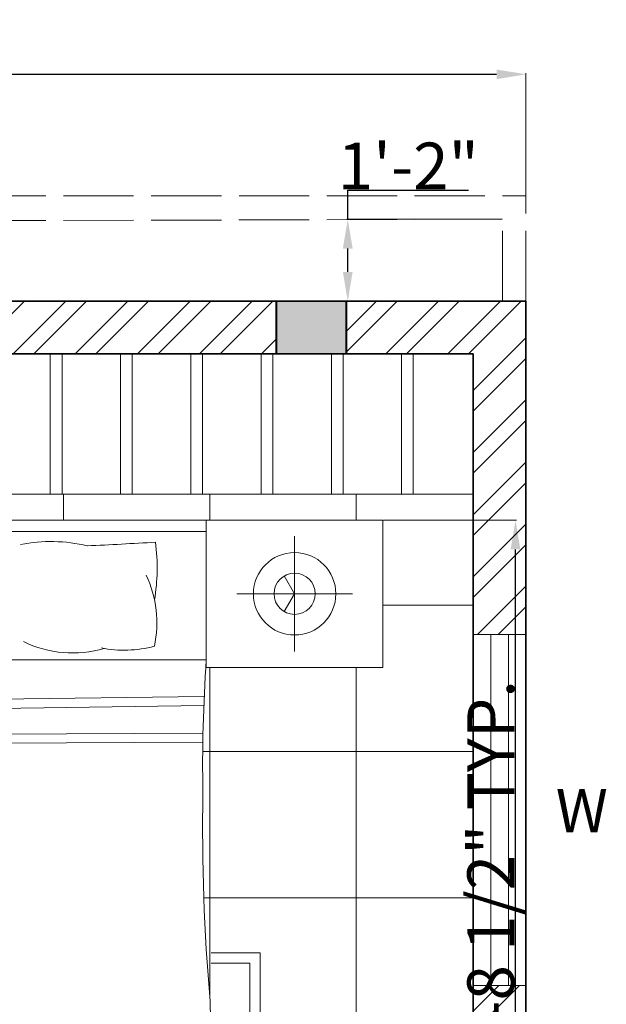
# Model space of a CAD drawing. Units: inches. Extents: x 351 to 1738, y -265 to 286.
# Tile 37 of 38: x 1480 to 1580, y 118 to 286. Entities that reach past the tile are written whole.
import ezdxf

# ---------------------------------------------------------------- set-up
doc = ezdxf.new("R2010")
doc.units = ezdxf.units.IN
doc.header["$MEASUREMENT"] = 0
doc.linetypes.add('ACAD_ISO02W100', pattern=[15, 12, -3])
for name, color, linetype, lineweight in [('A-ANNO-DIMS', 2, 'Continuous', 18), ('A-ANNO-SYMB', 7, 'Continuous', 18), ('A-COLS', 7, 'Continuous', 40), ('A-COLS-PATT', 6, 'Continuous', 13), ('A-FLOR-CASE', 9, 'Continuous', 18), ('A-FLOR-OVHD', 1, 'ACAD_ISO02W100', 18), ('A-FLOR-PATT', 9, 'Continuous', 9), ('A-FURN', 18, 'Continuous', 13), ('A-GLAZ', 4, 'Continuous', 18), ('A-WALL', 7, 'Continuous', 35), ('A-WALL-PATT', 152, 'Continuous', 13)]:
    doc.layers.add(name, color=color, linetype=linetype, lineweight=lineweight)
doc.styles.add('Annotative', font='arial.ttf')
doc.styles.get("Standard").update_dxf_attribs({"font": 'arial.ttf'})
doc.dimstyles.get("Standard").update_dxf_attribs({"dimtxt": 8, "dimasz": 5, "dimexe": 0.18, "dimexo": 0.0625, "dimgap": 0.09, "dimtad": 1, "dimtoh": 1, "dimzin": 0, "dimdsep": 46, "dimlunit": 4, "dimtxsty": 'Standard', "dimcen": 0, "dimclre": 256, "dimadec": 0, "dimazin": 0, "dimtfac": 1, "dimtofl": 0, "dimtmove": 0, "dimatfit": 3, "dimfxl": 1, "dimtolj": 1, "dimtzin": 0, "dimlwe": -1, "dimarcsym": 0})

# ---------------------------------------------------------------- blocks, each defined once
blk = doc.blocks.new('*D7')
at = {"layer": 'A-ANNO-DIMS', "color": 0, "transparency": 16777216}
for p, q in [((1034.7, 256.03), (1034.7, 276.92)), ((1566.7, 256.03), (1566.7, 276.92))]:
    blk.add_line(p, q, dxfattribs=at)
at = {"layer": 'A-ANNO-DIMS', "color": 0, "lineweight": -2, "transparency": 16777216}
blk.add_line((1039.7, 276.74), (1561.7, 276.74), dxfattribs=at)
at = {"layer": 'A-ANNO-DIMS', "color": 0, "transparency": 16777216}
for points in [[(1039.7, 277.57), (1039.7, 275.91), (1034.7, 276.74)], [(1561.7, 277.57), (1561.7, 275.91), (1566.7, 276.74)]]:
    blk.add_solid(points, dxfattribs=at)
at = {"layer": 'Defpoints', "color": 0, "transparency": 16777216}
for p in [(1566.7, 276.74), (1034.7, 255.96), (1566.7, 255.96)]:
    blk.add_point(p, dxfattribs=at)
at = {"layer": 'A-ANNO-DIMS', "color": 0, "transparency": 16777216, "insert": (1300.7, 280.83), "char_height": 8, "attachment_point": 5}
blk.add_mtext('\\A1;44\'-4"', dxfattribs=at)
blk = doc.blocks.new('*D9')
at = {"layer": 'A-ANNO-DIMS', "color": 0, "lineweight": -2, "transparency": 16777216}
for p, q in [((1536.28, 251.96), (1536.28, 256.96)), ((1536.28, 256.96), (1556.88, 256.96)), ((1536.28, 242.96), (1536.28, 246.96))]:
    blk.add_line(p, q, dxfattribs=at)
at = {"layer": 'A-ANNO-DIMS', "color": 0, "transparency": 16777216}
for p, q in [((1562.64, 251.96), (1536.1, 251.96)), ((1562.64, 237.96), (1536.1, 237.96))]:
    blk.add_line(p, q, dxfattribs=at)
for points in [[(1535.44, 246.96), (1537.11, 246.96), (1536.28, 251.96)], [(1535.44, 242.96), (1537.11, 242.96), (1536.28, 237.96)]]:
    blk.add_solid(points, dxfattribs=at)
at = {"layer": 'Defpoints', "color": 0, "transparency": 16777216}
for p in [(1536.28, 251.96), (1562.7, 251.96), (1562.7, 237.96)]:
    blk.add_point(p, dxfattribs=at)
at = {"layer": 'A-ANNO-DIMS', "color": 0, "transparency": 16777216, "insert": (1546.62, 261.07), "char_height": 8, "attachment_point": 5}
blk.add_mtext('\\A1;1\'-2"', dxfattribs=at)
blk = doc.blocks.new('BED-DOUBLE-W-NIGHTSTANDS')
for p, q in [((120.72, 126.39), (30.18, 126.39)), ((135.81, 105.9), (135.81, 125.61)), ((125.95, 115.76), (145.67, 115.76)), ((30.18, 104.48), (120.72, 104.48)), ((120.32, 98.22), (66.59, 97.46)), ((120.26, 96.67), (65.46, 95.89)), ((120.18, 91.92), (62.88, 91.69)), ((120.19, 90.37), (62.29, 90.13))]:
    blk.add_line(p, q)
for points in [[(30.18, 103.18), (0, 103.18), (0, 128.33), (150.9, 128.33), (150.9, 103.18), (120.72, 103.18), (120.72, 128.33)], [(134.05, 118.81), (135.81, 115.76), (134.05, 112.71)], [(121.56, 54.36), (129.93, 54.36), (129.93, 0), (19.92, 0), (19.92, 54.36), (28.45, 54.36)], [(28.45, 52.61), (21.67, 52.61), (21.67, 1.75), (128.18, 1.75), (128.18, 52.61), (121.53, 52.61)]]:
    blk.add_lwpolyline(points)
for points in [[(112.05, 124.57, -0.074897), (111.87, 114.71, 0.472817)], [(121.36, 46.14, 0.056112), (122.46, 37.83, 0.095341), (124.58, 29.84)]]:
    blk.add_lwpolyline(points, format="xyb")
for radius in [7.04, 3.52]:
    blk.add_circle((135.81, 115.76), radius)
for centre, radius, start, end in [((94.14, 98.17), 26.53, 76.3427, 101.1841), ((28.88, 1560.65), 1438.48, 272.85022, 273.31479), ((92.83, 110.76), 19.45, 348.2417, 24.8684), ((97.94, 124.85), 19.21, 243.8761, 286.1746), ((106.67, 126.34), 20.22, 258.9631, 284.8961), ((391.24, 86.04), 271.14, 176.1, 180.9282), ((473.78, 76.18), 353.69, 179.1145, 184.8735)]:
    blk.add_arc(centre, radius, start, end)
blk = doc.blocks.new('WARDROBE-PANELLED')
for p, q in [((101.27, 24), (101.27, 0)), ((103.27, 24), (103.27, 0)), ((113.27, 24), (113.27, 0)), ((115.27, 24), (115.27, 0)), ((125.27, 24), (125.27, 0)), ((127.27, 24), (127.27, 0)), ((137.27, 24), (137.27, 0)), ((139.27, 24), (139.27, 0)), ((149.27, 24), (149.27, 0)), ((151.27, 24), (151.27, 0)), ((161.27, 24), (161.27, 0)), ((163.27, 24), (163.27, 0)), ((0, 0), (173.5, 0))]:
    blk.add_line(p, q)
blk = doc.blocks.new('WIN-60')
for p, q in [((0, 6), (60, 6)), ((0, 3), (60, 3))]:
    blk.add_line(p, q)
blk.add_lwpolyline([(60, 0), (60, 9), (0, 9), (0, 0)], close=True)
blk = doc.blocks.new('*D47')
at = {"layer": 'A-ANNO-DIMS', "transparency": 16777216}
for p, q in [((1542.36, 200.52), (1565.11, 200.52)), ((1542.36, 72.19), (1565.11, 72.19))]:
    blk.add_line(p, q, dxfattribs=at)
at = {"layer": 'A-ANNO-DIMS', "color": 0, "lineweight": -2, "transparency": 16777216}
blk.add_line((1564.93, 77.19), (1564.93, 195.52), dxfattribs=at)
at = {"layer": 'A-ANNO-DIMS', "color": 0, "transparency": 16777216}
for points in [[(1564.1, 195.52), (1565.76, 195.52), (1564.93, 200.52)], [(1564.1, 77.19), (1565.76, 77.19), (1564.93, 72.19)]]:
    blk.add_solid(points, dxfattribs=at)
at = {"layer": 'Defpoints', "color": 0, "transparency": 16777216}
for p in [(1542.29, 200.52), (1564.93, 200.52), (1542.29, 72.19)]:
    blk.add_point(p, dxfattribs=at)
at = {"layer": 'A-ANNO-DIMS', "color": 0, "transparency": 16777216, "insert": (1560.7, 136.35), "char_height": 8, "attachment_point": 5, "rotation": 90}
blk.add_mtext('\\A1;10\'-8 1/2" TYP.', dxfattribs=at)

msp = doc.modelspace()

# ---------------------------------------------------------------- hatches: boundary and pattern name
at = {"layer": 'A-COLS-PATT'}
h = msp.add_hatch(color=256, dxfattribs=at)
h.dxf.hatch_style = 1
h.paths.add_polyline_path([(1112.704, 237.963), (1103.704, 237.963), (1103.704, 228.963), (1112.704, 228.963)])
h.paths.add_polyline_path([(1115.704, 237.963), (1112.704, 237.963), (1112.704, 228.963), (1115.704, 228.963)])
h.paths.add_polyline_path([(1043.704, 255.963), (1034.704, 255.963), (1034.704, 243.963), (1043.704, 243.963)])
h.paths.add_polyline_path([(1043.704, 210.963), (1034.704, 210.963), (1034.704, 198.963), (1043.704, 198.963)])
h.paths.add_polyline_path([(1043.704, -45.037), (1034.704, -45.037), (1034.704, -57.037), (1043.704, -57.037)])
h.paths.add_polyline_path([(1112.704, -45.037), (1103.704, -45.037), (1103.704, -57.037), (1112.704, -57.037)])
h.paths.add_polyline_path([(1112.704, -161.037), (1103.704, -161.037), (1103.704, -164.037), (1103.704, -173.037), (1112.704, -173.037)])
h.paths.add_polyline_path([(1043.704, -161.037), (1034.704, -161.037), (1034.704, -173.037), (1043.704, -173.037)])
h.paths.add_polyline_path([(1248.549, -164.037), (1236.549, -164.037), (1236.549, -173.037), (1248.549, -173.037)])
h.paths.add_polyline_path([(1248.549, -50), (1236.549, -50), (1236.549, -59), (1248.549, -59)])
h.paths.add_polyline_path([(1248.704, 73.463), (1244.704, 73.463), (1244.704, 64.463), (1248.704, 64.463)])
h.paths.add_polyline_path([(1244.704, 73.463), (1236.704, 73.463), (1236.704, 64.463), (1244.704, 64.463)])
h.paths.add_polyline_path([(1248.704, 237.963), (1236.704, 237.963), (1236.704, 228.963), (1248.704, 228.963)])
h.paths.add_polyline_path([(1392.204, 237.963), (1380.204, 237.963), (1380.204, 228.963), (1392.204, 228.963)])
h.paths.add_polyline_path([(1536.064, 237.963), (1524.064, 237.963), (1524.064, 228.963), (1536.064, 228.963)])
h.paths.add_polyline_path([(1536.064, 73.463), (1524.064, 73.463), (1524.064, 64.463), (1536.064, 64.463)])
h.paths.add_polyline_path([(1384.204, 73.463), (1380.204, 73.463), (1380.204, 64.463), (1384.204, 64.463)])
h.paths.add_polyline_path([(1392.064, 73.463), (1384.204, 73.463), (1384.204, 64.463), (1392.064, 64.463)])
h.paths.add_polyline_path([(1536.064, -53.037), (1524.064, -53.037), (1524.064, -57.037), (1536.064, -57.037)])
h.paths.add_polyline_path([(1536.064, -48.037), (1524.064, -48.037), (1524.064, -53.037), (1536.064, -53.037)])
h.paths.add_polyline_path([(1392.064, -48.037), (1380.064, -48.037), (1380.064, -56.5), (1380.065, -57.037), (1392.064, -57.037)])
h.paths.add_polyline_path([(1536.064, -164.037), (1524.064, -164.037), (1524.064, -173.037), (1536.064, -173.037)])
at = {"layer": 'A-FLOR-PATT', "transparency": 33554559}
h = msp.add_hatch(dxfattribs=at)
h.set_pattern_fill('ANSI37', color=256, scale=200, angle=135)
h.set_pattern_definition([(180, (1112.704, -164.037), (-2e-15, -25), []), (270, (1112.704, -164.037), (25, -5e-15), [])])
h.paths.add_polyline_path([(1380.064, 73.463), (1380.132, 148.463), (1338.064, 148.463), (1290.704, 148.463), (1290.704, 88.463), (1248.704, 88.463), (1248.704, -2.009), (1244.704, -2.009), (1244.704, 142.457), (1160.704, 142.457), (1160.704, 158.963), (1160.704, 170.137), (1160.704, 206.137), (1160.704, 228.963), (1112.704, 228.963), (1112.704, 209.963), (1112.704, 168.963), (1124.704, 168.963), (1124.704, 162.963), (1112.704, 162.963), (1112.704, 64.463), (1112.704, 60.463), (1112.704, 0.463), (1112.704, -48.026), (1146.804, -47.981), (1146.804, -35.691), (1207.804, -35.691), (1207.804, -47.902), (1236.542, -47.864), (1236.544, -50.009), (1248.5, -50.009), (1248.506, -102.915), (1248.512, -150.915), (1248.514, -164.037), (1248.549, -164.037), (1273.017, -164.037), (1273.017, -128.799), (1355.24, -128.799), (1355.24, -164.037), (1384.204, -164.037), (1384.204, -57.037), (1380.064, -57.037), (1380.064, -48.037), (1392.064, -48.037), (1392.064, -53.037), (1406.549, -53.037), (1406.549, -57.037), (1401.204, -57.037), (1401.204, -147.037), (1468.204, -147.037), (1468.204, -138.5), (1472.204, -138.5), (1472.204, -102.5), (1468.204, -102.5), (1468.204, -57.037), (1442.549, -57.037), (1442.549, -53.037), (1463.049, -53.037), (1463.049, -40.747), (1524.049, -40.747), (1524.049, -48.037), (1536.064, -48.037), (1536.064, -53.037), (1557.704, -53.037), (1557.704, 204.963), (1384.204, 204.963), (1384.204, 73.463), (1392.064, 73.463), (1392.064, 64.463), (1384.204, 64.463), (1384.204, -3.5), (1380.204, -3.537), (1380.204, 64.463), (1380.064, 64.463)])
h.paths.add_polyline_path([(1510.714, 86.458, -0.1039845), (1511.661, 85.595, 0.4704384), (1510.158, 87.614, 0.0961001)], flags=16)
h.paths.add_polyline_path([(1510.443, 100.266, 0.009798), (1504.693, 100.48, 0.0287898), (1504.6, 99.767, -0.1653311), (1505.519, 96.135, -0.1436014)], flags=16)
h.paths.add_polyline_path([(1487.201, 85.595, -0.1039845), (1488.148, 86.458, 0.0961001), (1488.704, 87.614, 0.4704384)], flags=0)
h.paths.add_polyline_path([(1495.052, 100.43), (1494.178, 100.43, -0.0264629), (1494.262, 99.774, -0.1442193)], flags=16)
h.paths.add_polyline_path([(1444.485, 86.458, -0.1039845), (1445.433, 85.595, 0.4704384), (1443.93, 87.614, 0.0961001)], flags=16)
h.paths.add_polyline_path([(1420.972, 85.595, -0.1039845), (1421.92, 86.458, 0.0961001), (1422.475, 87.614, 0.4704384)], flags=16)
h.paths.add_polyline_path([(1428.632, 100.335, 0.0010541), (1427.971, 100.309, -0.0215241), (1428.033, 99.774, -0.1143008)], flags=16)
h.paths.add_polyline_path([(1419.906, 143.708, 0.0249793), (1420.222, 157.526), (1421.573, 159.101), (1421.573, 175.369), (1391.393, 175.369), (1391.393, 200.519), (1542.294, 200.519), (1542.294, 175.369), (1512.028, 175.369, 0.0198653), (1511.521, 153.838, 0.0251335), (1512.758, 118.323, 0.0205529), (1512.942, 115.253), (1419.834, 115.253, -0.0004142), (1419.843, 124.798), (1413.059, 124.798), (1413.059, 84.437, -0.0618528), (1415.831, 80.45, -0.0930773), (1420.972, 85.595, -0.2675367), (1422.371, 84.732, 0.0851103), (1424.052, 84.616, -0.8853927), (1424.033, 84.851, -1.1258145), (1424.073, 84.366, -0.0879871), (1422.371, 84.732, -0.2675367), (1422.326, 83.089, -0.3705421), (1420.972, 85.595, 0.0930773), (1415.831, 80.45, -0.0874142), (1417.914, 73.937), (1418.941, 73.937, 0.0272504), (1418.913, 76.906, -0.1157032), (1421.051, 73.937), (1445.354, 73.937, -0.1157032), (1447.492, 76.906, 0.0272504), (1447.464, 73.937), (1448.491, 73.937, -0.0874142), (1450.574, 80.45, 0.0930773), (1445.433, 85.595, -0.3705421), (1444.079, 83.089, -0.2675367), (1444.034, 84.732, -0.0879871), (1442.332, 84.366, -1.1258145), (1442.372, 84.851, -2.0327363), (1442.364, 84.368, 0.0863779), (1444.034, 84.732, -0.2675367), (1445.433, 85.595, -0.0930773), (1450.574, 80.45, -0.2577317), (1466.483, 90.927, -0.4786702), (1468.832, 91.907, -0.4786702), (1471.18, 90.927, -0.26264), (1483.053, 81.78, -0.0718662), (1487.201, 85.595, -0.2675367), (1488.6, 84.732, 0.0851103), (1490.28, 84.616, -0.8853927), (1490.262, 84.851, -1.1258145), (1490.301, 84.366, -0.0879871), (1488.6, 84.732, -0.2675367), (1488.554, 83.089, -0.3705421), (1487.201, 85.595, 0.0718662), (1483.053, 81.78, -0.1320648), (1484.143, 73.937), (1485.169, 73.937, 0.0272504), (1485.142, 76.906, -0.1157032), (1487.28, 73.937), (1511.582, 73.937, -0.1157032), (1513.72, 76.906, 0.0272504), (1513.693, 73.937), (1514.719, 73.937, -0.0874142), (1516.802, 80.45, 0.0930773), (1511.661, 85.595, -0.3705421), (1510.308, 83.089, -0.2675367), (1510.262, 84.732, -0.0879871), (1508.561, 84.366, -1.1258145), (1508.601, 84.851, -2.0327363), (1508.592, 84.368, 0.0863779), (1510.262, 84.732, -0.2675367), (1511.661, 85.595, -0.0930773), (1516.802, 80.45, -0.0618528), (1519.575, 84.437), (1519.575, 73.937), (1413.059, 73.937), (1413.059, 124.798), (1419.843, 124.798, -0.0008205)], flags=16)
h.paths.add_polyline_path([(1220.149, 54.133, -0.1039845), (1220.869, 53.476, 0.4704384), (1219.727, 55.011, 0.0961001)], flags=16)
h.paths.add_polyline_path([(1219.944, 64.626, 0.009798), (1215.574, 64.789, 0.0287898), (1215.503, 64.247, -0.1653311), (1216.201, 61.487, -0.1436014)], flags=16)
h.paths.add_polyline_path([(1209.779, 64.449, 0.0974459), (1209.339, 64.751), (1208.247, 64.751, 0.1273905), (1207.7, 64.326, 0.1715858), (1206.95, 61.475, -0.1588542), (1207.636, 59.45, 0.0158984), (1207.795, 59.218, 0.0615457), (1208.598, 59.616, 0.1754158), (1208.638, 60.099, -0.2847793), (1209.348, 62.472, 0.3262165)], flags=16)
h.paths.add_polyline_path([(1169.818, 54.133, -0.1039845), (1170.538, 53.476, 0.4704384), (1169.396, 55.011, 0.0961001)], flags=16)
h.paths.add_polyline_path([(1159.017, 62.472, 0.2847642), (1158.307, 60.099, -0.1754332), (1158.267, 59.616, 0.3929302), (1159.448, 64.449, -0.3262298)], flags=16)
h.paths.add_polyline_path([(1156.342, 58.239, -0.1783213), (1154.011, 55.31, -0.1747359), (1154.722, 55.233, -0.2008015), (1156.27, 56.086, 0.1269899), (1157.283, 58.991, -0.0912053)], flags=16)
h.paths.add_polyline_path([(1156.624, 61.413, 0.1572752), (1157.316, 64.247, 0.1696217)], flags=16)
h.paths.add_polyline_path([(1152.67, 54.133, -0.0961001), (1151.95, 53.476, 0.0640762), (1154.465, 54.384, 0.1990158)], flags=16)
h.paths.add_polyline_path([(1202.281, 53.476, -0.1039845), (1203, 54.133, 0.0961001), (1203.423, 55.011, 0.4704384)], flags=0)
h.paths.add_polyline_path([(1151.139, 97.64, 0.0249793), (1151.379, 108.141), (1152.406, 109.338), (1152.406, 121.701), (1129.47, 121.701), (1129.47, 140.814), (1244.149, 140.814), (1244.149, 121.701), (1221.148, 121.701, 0.0198653), (1220.763, 105.338, 0.0251335), (1221.703, 78.349, 0.0205529), (1221.843, 76.016), (1151.078, 76.016, -0.1287433), (1148.786, 65.037, 0.5393525), (1150.327, 64.171, -0.027594), (1163.481, 64.751, 0.0976954), (1163.04, 64.449, 0.3262165), (1163.471, 62.472, -0.2847765), (1164.181, 60.099, -0.1947567), (1165.846, 61.443, -0.1554021), (1165.172, 64.247, -0.1660224), (1165.869, 61.475, -0.1770142), (1167.852, 62.77, -0.4482027), (1169.974, 60.807, -0.3934987), (1167.679, 57.86, -0.8955483), (1168.438, 54.524, -0.3557668), (1166.218, 56.086, -0.066024), (1165.505, 57.539), (1165.251, 56.243, -0.3717324), (1164.02, 59.758, -0.3736141), (1163.04, 64.449, -0.0976954), (1163.481, 64.751, 0.0213538), (1153.294, 64.429, -0.1341826), (1156.695, 61.368, 0.1868727), (1154.636, 62.77, 0.4482027), (1152.514, 60.807, 0.4037263), (1154.905, 57.846, 0.7112192), (1153.334, 55, 0.5315397), (1151.95, 53.476, -0.2675367), (1153.013, 52.821, 0.0851103), (1154.29, 52.732, -0.8853927), (1154.276, 52.911, -1.1258145), (1154.306, 52.543, -0.0879871), (1153.013, 52.821, -0.2675367), (1152.978, 51.572, -0.3705421), (1151.95, 53.476, 0.0930773), (1148.043, 49.566, -0.0874142), (1149.626, 44.617), (1150.406, 44.617, 0.0272504), (1150.385, 46.873, -0.1157032), (1152.01, 44.617), (1170.478, 44.617, -0.1157032), (1172.103, 46.873, 0.0272504), (1172.082, 44.617), (1172.862, 44.617, -0.0874142), (1174.445, 49.566, 0.0930773), (1170.538, 53.476, -0.3705421), (1169.51, 51.572, -0.2675367), (1169.475, 52.821, -0.0879871), (1168.182, 52.543, -1.1258145), (1168.212, 52.911, -2.0327363), (1168.206, 52.544, 0.0863779), (1169.475, 52.821, -0.2675367), (1170.538, 53.476, -0.0930773), (1174.445, 49.566, -0.2577317), (1186.536, 57.528, -0.4786702), (1188.321, 58.273, -0.4786702), (1190.106, 57.528, -0.26264), (1199.128, 50.577, -0.0718662), (1202.281, 53.476, -0.2675367), (1203.344, 52.821, 0.0851103), (1204.621, 52.732, -0.8853927), (1204.607, 52.911, -1.1258145), (1204.637, 52.543, -0.0879871), (1203.344, 52.821, -0.2675367), (1203.309, 51.572, -0.3705421), (1202.281, 53.476, 0.0718662), (1199.128, 50.577, -0.1320648), (1199.957, 44.617), (1200.737, 44.617, 0.0272504), (1200.716, 46.873, -0.1157032), (1202.341, 44.617), (1220.809, 44.617, -0.1157032), (1222.434, 46.873, 0.0272504), (1222.413, 44.617), (1223.193, 44.617, -0.0874142), (1224.776, 49.566, 0.0930773), (1220.869, 53.476, -0.3705421), (1219.841, 51.572, -0.2675367), (1219.806, 52.821, -0.0879871), (1218.513, 52.543, -1.1258145), (1218.543, 52.911, -2.0327363), (1218.537, 52.544, 0.0863779), (1219.806, 52.821, -0.2675367), (1220.869, 53.476, -0.0930773), (1224.776, 49.566, -0.0618528), (1226.883, 52.597), (1226.883, 44.617), (1145.936, 44.617), (1145.936, 83.269), (1151.091, 83.269, -0.0008205)], flags=16)
h.paths.add_polyline_path([(1218.01, 57.86, -0.8955483), (1218.769, 54.524, -0.3557668), (1216.549, 56.086, -0.066024), (1215.836, 57.539), (1215.582, 56.243, -0.3717324), (1214.351, 59.758, -0.3736141), (1213.371, 64.449, 0.3262165), (1213.802, 62.472, -0.2847765), (1214.512, 60.099, -0.1947567), (1216.177, 61.443, -0.1799907), (1218.183, 62.77, -0.4482027), (1220.305, 60.807, -0.3934987)], flags=16)
h.paths.add_polyline_path([(1424.735, 91.363, -0.3934987), (1421.715, 95.241, -0.4482027), (1424.507, 97.824, -0.1799907), (1427.147, 96.077, -0.1947567), (1429.338, 94.309, -0.2847765), (1430.272, 97.432, 0.3262165), (1430.839, 100.034, -0.3736141), (1429.55, 93.861, -0.3717324), (1427.929, 89.235), (1427.596, 90.941, -0.066024), (1426.657, 89.029, -0.3557668), (1423.736, 86.973, -0.8955483)], flags=16)
h.paths.add_polyline_path([(1238.033, 131.257, -1), (1227.329, 131.257, -1)], flags=0)
h.paths.add_polyline_path([(1235.357, 131.257, -1), (1230.005, 131.257, -1)], flags=0)
h.paths.add_polyline_path([(1214.039, 54.243, 0.1543819), (1214.38, 53.992, 0.3589549), (1213.613, 54.016, 0.6039484), (1214.379, 53.657, 0.3713191), (1213.968, 52.872, 0.1879935), (1214.312, 52.809, -0.592455), (1213.953, 52.967, -0.2942791), (1214.083, 53.691, -1.3001871), (1213.881, 54.134, -0.2837621), (1214.469, 53.896, 1.1509396)], flags=16)
h.paths.add_polyline_path([(1212.091, 56.286, -0.4084338), (1211.337, 56.445, -0.0362594), (1211.098, 56.848, -0.2360976), (1211.59, 56.63, 0.0353445), (1211.835, 56.543, -0.4752408), (1212.091, 56.286, -0.4752408), (1212.438, 56.182, 0.0353445), (1212.631, 56.007, -0.2360976), (1213.056, 55.676, -0.0362594), (1212.588, 55.697, -0.4084338)], flags=16)
h.paths.add_polyline_path([(1211.469, 50.297, 0.296043), (1210.47, 50.527, 0.310883), (1211.931, 50.148, 0.0212546)], flags=16)
h.paths.add_polyline_path([(1213.739, 51.818, -0.0362594), (1213.271, 51.838, -0.4084337), (1212.774, 52.427, -0.0947856), (1212.293, 50.703, 1.1504738), (1212.911, 50.232, 0.1662877), (1213.265, 50.68, -0.0252543), (1212.603, 50.13, 1.0879317), (1212.471, 49.407, 0.1662877), (1213.02, 49.251, -0.016128), (1212.567, 49.563, -0.286859), (1212.217, 49.638, 0.0221563), (1212.046, 50.055, -0.6461302), (1212.185, 50.498, 0.0884116), (1212.732, 52.077, -1.1860374), (1213.121, 52.323, 0.0353445), (1213.314, 52.148, -0.2360976)], flags=16)
h.paths.add_polyline_path([(1212.094, 50.342, -0.0485241), (1211.54, 49.605, -1.1038339), (1211.397, 48.738, -0.7855147), (1211.683, 48.254, -0.3920429), (1210.948, 48.525, -0.3928194), (1210.561, 47.995, -0.592455), (1210.201, 48.153, -0.2942791), (1210.331, 48.877, -0.7041716), (1210.316, 49.592, -0.6793441), (1210.729, 50.112, 0.5636764)], flags=16)
h.paths.add_polyline_path([(1211.274, 49.829, -0.1398258), (1210.745, 49.859, -0.2178785), (1210.948, 49.509, -0.4985724)], flags=0)
h.paths.add_polyline_path([(1433.426, 81.49, -0.181571), (1434.245, 81.788, -0.0080665), (1433.726, 82.205, 0.0455784), (1432.755, 81.242, 0.1790113)], flags=16)
h.paths.add_polyline_path([(1434.146, 81.009, -0.1324418), (1433.645, 80.771, 0.2590893), (1433.234, 80.471, -0.1802109), (1433.392, 80.805, -0.1699398), (1432.758, 81.109, 0.0326525), (1433.273, 80.474, -0.4933627), (1434.046, 80.146, -0.3904966)], flags=16)
h.paths.add_polyline_path([(1434.83, 80.047, -0.9475376), (1435.294, 79.576, -0.2991282), (1434.625, 79.404, -0.2704392), (1435.01, 78.591, -0.592455), (1434.537, 78.382, -0.3928194), (1434.027, 79.08, -0.3920429), (1433.06, 78.723, -0.3520423), (1433.003, 79.197, -0.1972159), (1433.75, 79.734, -0.7136405), (1434.447, 79.939, -0.2147903), (1434.819, 80.475, 0.4088333), (1435.075, 80.803, -0.2261519)], flags=16)
h.paths.add_polyline_path([(1432.67, 81.217, -0.4542182), (1431.897, 79.923, -0.4144105), (1431.301, 80.035, 0.0161291), (1431.897, 80.445, 0.2795702), (1432.073, 80.871, -0.2895037), (1431.103, 81.321, -0.4144105), (1430.978, 81.915, 0.0161296), (1431.586, 81.521, 0.341293), (1432.125, 81.583, -0.8131856)], flags=16)
h.paths.add_polyline_path([(1429.893, 86.381, -0.9475376), (1430.358, 85.91, -0.1731062), (1429.984, 85.712, -0.0388172), (1431.625, 84.214, -0.0879005), (1432.097, 88.549, -0.0497684), (1431.254, 88.49, -0.2360976), (1431.814, 88.925, 0.0353445), (1432.067, 89.155, -0.4752408), (1432.524, 89.291, -0.4752408), (1432.86, 89.63, 0.0353445), (1433.182, 89.744, -0.2360976), (1433.83, 90.032, -0.0362594), (1433.516, 89.502, -0.4084338), (1432.524, 89.291, -0.3124239), (1432.106, 88.58, 0.0885594), (1431.625, 84.214, -0.4084337), (1430.971, 83.439, -0.0362594), (1430.355, 83.412, -0.2360976), (1430.914, 83.847, 0.0353445), (1431.168, 84.078, -0.4752408), (1431.625, 84.214, 0.0388172), (1429.984, 85.712, -0.3217316), (1429.333, 86.048, -0.32743), (1429.883, 86.809, 0.4088333), (1430.138, 87.138, -0.2261519)], flags=16)
h.paths.add_polyline_path([(1211.206, 58.616, -0.9997836), (1211.336, 59.323, -0.6149935)], flags=16)
h.paths.add_polyline_path([(1210.288, 49.429, 0.1543819), (1210.629, 49.178, 0.3589549), (1209.861, 49.202, 0.6039484), (1210.627, 48.843, -0.5348247), (1210.806, 49.295, 0.7483464)], flags=16)
h.paths.add_polyline_path([(1209.589, 51.828, -0.0087906), (1209.775, 51.753, 0.1122315), (1209.466, 52.019, 1.4188509), (1209.014, 51.708, -0.4587257), (1208.651, 51.073, -0.592455), (1208.291, 51.232, -0.2942791), (1208.421, 51.955, -1.3001871), (1208.219, 52.398, -0.2260052), (1208.719, 52.257, -0.4755189), (1209.158, 52.369, -1.4554994), (1209.603, 52.664, 0.4213049), (1209.191, 52.262, -0.5912116), (1208.979, 51.796, 0.4973986), (1209.773, 51.333, 0.6493116)], flags=16)
h.paths.add_polyline_path([(1208.029, 52.041, 0.5446671), (1208.832, 52.045, 0.220132)], flags=0)
h.paths.add_polyline_path([(1210.438, 51.425, -0.2041997), (1210.277, 52.018, 0.2708262), (1209.915, 52.897, 0.3241145)], flags=0)
h.paths.add_polyline_path([(1209.668, 52.407, -0.60139), (1208.99, 52.221, -0.3949159), (1208.248, 52.83, -0.8367916), (1208.651, 53.017, -0.3384876), (1209.039, 52.571, 0.1941379), (1209.191, 52.262, 0.4139945), (1209.712, 52.475, 0.5177103), (1210.503, 51.416, 0.401922), (1209.493, 50.93, 0.2063956), (1209.516, 50.165, -0.3194629), (1210.417, 51.418, -0.466635)], flags=16)
h.paths.add_polyline_path([(1206.601, 56.086, -0.3557668), (1204.381, 54.524, -0.9211983), (1205.236, 57.846, 0.2065693), (1207.614, 58.991, -0.1269899)], flags=16)
h.paths.add_polyline_path([(1435.487, 82.816, 0.5277653), (1436.615, 83.361, 0.5085402), (1437.05, 82.433, 0.592455), (1437.524, 82.641, 0.3312448), (1436.963, 83.548, 0.3878632), (1437.808, 83.626, 0.5929544), (1437.618, 84.176, 0.2260158), (1436.961, 83.99, 0.3182053), (1437.588, 84.854, 0.6893744), (1437.05, 84.991, 0.3357648), (1436.539, 84.41, -0.1569934), (1436.404, 84.065, -0.4346112), (1436.961, 83.99, -0.2147903), (1437.333, 84.526, 0.4088333), (1437.588, 84.854, -0.2261519), (1437.343, 84.097, -0.9475376), (1437.808, 83.626, -0.2991282), (1437.139, 83.455, -0.2704392), (1437.524, 82.641, -0.592455), (1437.05, 82.433, -0.3928194), (1436.541, 83.13, -0.4396601), (1435.475, 82.794, -0.174614), (1435.942, 82.244, -0.2063956), (1435.912, 81.237, -0.2708262), (1435.125, 82.208, 0.2079765), (1434.686, 82.904, -0.1964955)], flags=16)
h.paths.add_polyline_path([(1435.386, 84.832, 0.270811), (1434.91, 83.676, -0.2042174), (1434.699, 82.895, 0.3241145)], flags=0)
h.paths.add_polyline_path([(1435.68, 84.18, -0.2176564), (1435.554, 83.304, -0.1767045), (1436.236, 83.778, -0.3730364)], flags=0)
h.paths.add_polyline_path([(1435.566, 100.034, 0.3262165), (1436.133, 97.432, -0.2847765), (1437.067, 94.309, -0.1947567), (1439.258, 96.077, -0.1554021), (1438.371, 99.767, -0.1660224), (1439.289, 96.12, -0.1770142), (1441.897, 97.824, -0.4482027), (1444.69, 95.241, -0.3934987), (1441.67, 91.363, -0.8955483), (1442.669, 86.973, -0.3557668), (1439.748, 89.029, -0.066024), (1438.809, 90.941), (1438.476, 89.235, -0.3717324), (1436.855, 93.861, -0.3736141)], flags=16)
h.paths.add_polyline_path([(1191.252, 49.507, -0.2740221), (1190.658, 48.409, 0.2675367), (1191.311, 47.344, 0.3705421)], flags=0)
h.paths.add_polyline_path([(1190.301, 49.717, 0.1990158), (1188.619, 49.04, 0.0640762), (1191.252, 49.507, -0.0961001)], flags=0)
h.paths.add_polyline_path([(1189.518, 47.857, 1.1258145), (1189.676, 47.523, 2.0446052)], flags=0)
h.paths.add_polyline_path([(1464.974, 80.372, 0.2740221), (1465.756, 78.927, -0.0830131)], flags=0)
h.paths.add_polyline_path([(1464.974, 80.372, 0.3705421), (1464.897, 77.525, 0.5763244)], flags=0)
h.paths.add_polyline_path([(1464.974, 80.372, -0.4704384), (1467.284, 81.372, -0.0961001), (1466.226, 80.648, -0.1990158), (1468.439, 79.757, -0.0640762)], flags=0)
h.paths.add_polyline_path([(1189.511, 56.43, -0.2594668), (1188.321, 56.391, -0.2594668), (1187.13, 56.43, 0.0851103), (1188.193, 55.716, -0.8853927), (1188.27, 55.878, -1.1960133), (1188.355, 55.442, 0.1014587)], flags=0)
h.paths.add_polyline_path([(1188.321, 57.596, 0.0780722), (1187.678, 57.24, 0.0155503), (1188.321, 57.136, 0.0155503), (1188.964, 57.24, 0.0780722)], flags=0)
h.paths.add_polyline_path([(1190.164, 55.365, -0.5763244), (1190.106, 57.528, -0.1982945), (1188.321, 58.319, -0.1982945), (1186.536, 57.528, -0.5763244), (1186.477, 55.365, -0.3705421), (1186.536, 57.528, 0.1982945), (1188.321, 58.319, 0.1982945), (1190.106, 57.528, -0.3705421)], flags=0)
h.paths.add_polyline_path([(1188.372, 55.878, 1.1258145), (1188.529, 55.544, 2.0446052)], flags=0)
h.paths.add_polyline_path([(1186.341, 49.717, -0.0961001), (1185.389, 49.507, 0.0640762), (1188.022, 49.04, 0.1990158)], flags=0)
h.paths.add_polyline_path([(1185.389, 49.507, -0.2675367), (1185.984, 48.409, 0.0851103), (1187.046, 47.695, -0.8853927), (1187.123, 47.857, -1.1258145), (1186.966, 47.523, -0.0879871), (1185.984, 48.409, -0.2675367), (1185.331, 47.344, -0.3705421)], flags=0)
h.paths.add_polyline_path([(1399.441, 187.944, -1), (1413.525, 187.944, -1)], flags=0)
h.paths.add_polyline_path([(1402.962, 187.944, -1), (1410.004, 187.944, -1)], flags=0)
h.paths.add_polyline_path([(1357.663, -72.245), (1377.272, -72.245), (1377.272, -91.854), (1357.663, -91.854)], flags=16)
h.paths.add_polyline_path([(1467.256, 78.201, -1.1258145), (1467.049, 77.761, -2.0446052)], flags=0)
h.paths.add_polyline_path([(1468.822, 88.714, 0.9411249), (1469.106, 88.316, 1.1371523), (1468.765, 88.755, 0.890986), (1468.99, 88.245, 0.0948283), (1470.398, 89.481, -0.2675367), (1471.18, 90.927, -0.0281232), (1469.678, 90.547, -0.0287737), (1469.948, 90.311, -0.0203267), (1468.832, 90.41, -0.0203267), (1467.716, 90.311, -0.0287737), (1467.986, 90.547, -0.0281232), (1466.483, 90.927, -0.2675367), (1467.265, 89.481, 0.0851103), (1468.663, 88.542, -1.2023159)], flags=0)
h.paths.add_polyline_path([(1178.25, 124.523, -0.1199286), (1165.65, 124.145, -0.1073492), (1159.133, 124.446, -0.1028906), (1159.132, 130.465, -0.0748968), (1158.993, 137.956, 0.002027), (1167.844, 137.479, -0.07553), (1180.337, 137.666, -0.0758613), (1186.502, 137.688, -0.1409896), (1186.272, 130.046, -0.0954805), (1186.729, 124.748, -0.10603)], flags=0)
h.paths.add_polyline_path([(1469.225, 79.757, -0.1990158), (1471.437, 80.648, -0.0961001), (1470.379, 81.372, -0.4704384), (1472.689, 80.372, -0.3705421), (1472.766, 77.525, -0.2675367), (1471.907, 78.927, -0.0879863), (1470.615, 77.761, -1.1258491), (1470.408, 78.201, -2.0327363), (1470.642, 77.778, 0.0863779), (1471.907, 78.927, -0.2675367), (1472.689, 80.372, -0.0640762)], flags=0)
h.paths.add_polyline_path([(1430.423, 186.902, -0.0748968), (1430.24, 196.758, 0.002027), (1441.887, 196.131, -0.07553), (1458.326, 196.377, -0.0758613), (1466.438, 196.406, -0.1409896), (1466.136, 186.35, -0.0954805), (1466.737, 179.378, -0.10603), (1455.58, 179.082, -0.1199286), (1439, 178.585, -0.1073492), (1430.425, 178.981, -0.1028906)], flags=0)
h.paths.add_polyline_path([(1162.258, 49.939, 0.3357645), (1161.87, 49.497, -0.1569936), (1161.767, 49.235, -0.4346112), (1162.19, 49.178, -0.2147903), (1162.473, 49.585, 1.5291948)], flags=16)
h.paths.add_polyline_path([(1161.683, 49.021, 0.5815181), (1161.268, 49.583, 0.5927609)], flags=16)
h.paths.add_polyline_path([(1162.602, 48.058, 0.3713191), (1162.192, 48.843, 0.4345332), (1162.88, 48.962, 0.1850806), (1162.197, 48.926, 1.1218369)], flags=16)
h.paths.add_polyline_path([(1161.443, 48.941, -1.3071038), (1161.495, 48.571, -0.2177521), (1161.136, 48.254, 0.6973029), (1161.871, 49.048, 0.1215141)], flags=16)
h.paths.add_polyline_path([(1162.531, 49.429, -0.2070837), (1162.05, 49.146, -0.9920299)], flags=16)
h.paths.add_polyline_path([(1161.304, 49.578, -0.7196675), (1161.513, 50.079, -0.1304275), (1160.836, 50.168, 0.0395926)], flags=0)
h.paths.add_polyline_path([(1162.036, 50.584, -0.0080665), (1161.642, 50.9, 0.0293675), (1161.35, 50.297, -0.2057884)], flags=16)
h.paths.add_polyline_path([(1162.882, 51.392, -0.1247327), (1162.763, 51.828, -0.1011907), (1162.399, 51.438, -0.153425)], flags=0)
h.paths.add_polyline_path([(1164.235, 51.85, -0.3091075), (1164.513, 51.136, -0.6271245), (1163.781, 51.603, -0.6859091), (1162.777, 51.219, -0.2332851), (1163.303, 50.165, -0.2708262), (1162.705, 50.903, 0.2041997), (1162.381, 51.425, 0.204182), (1162.542, 52.018, -0.2708414), (1162.903, 52.897, -0.1272607), (1163.219, 52.529, -1.1686811), (1163.781, 52.587, -0.3291117), (1164.168, 53.017, -0.8367917), (1164.571, 52.83, -0.1933406), (1164.391, 52.338, -0.9475376), (1164.744, 51.981, -0.2991282)], flags=16)
h.paths.add_polyline_path([(1163.598, 51.937, -1.2629561), (1163.236, 51.831, 0.0125754), (1162.971, 51.721, 0.2306566), (1163.151, 52.407, -0.1648982), (1163.178, 52.661, -0.4493201), (1163.628, 52.262, -0.721477), (1164.154, 52.088, -0.8499982)], flags=0)
h.paths.add_polyline_path([(1161.613, 58.616, -0.9804131), (1161.525, 59.049, -2.9089348)], flags=16)
h.paths.add_polyline_path([(1160.252, 49.166, -0.4144105), (1159.799, 49.251, 0.0161291), (1160.252, 49.563, 0.2795702), (1160.386, 49.887, -0.2895037), (1159.649, 50.229, -0.4144105), (1159.554, 50.68, 0.0161296), (1160.015, 50.381, 0.6178854), (1160.526, 50.703, -0.0947856), (1160.045, 52.427, -0.1404436), (1159.682, 52.042, -0.0578559), (1159.3, 51.872, 0.5448433), (1160.046, 52.419, -0.0881216), (1160.404, 55.721, -0.0497684), (1159.763, 55.676, -0.2360976), (1160.188, 56.007, 0.0353445), (1160.381, 56.182, -0.4752408), (1160.728, 56.286, -0.4752408), (1160.984, 56.543, 0.0353445), (1161.229, 56.63, -0.2360976), (1161.721, 56.848, -0.0362594), (1161.482, 56.445, -0.4084338), (1160.728, 56.286, -0.3124239), (1160.411, 55.745, 0.0885594), (1160.045, 52.427, 0.1070813), (1160.634, 50.498, -0.4947977), (1160.839, 50.149, -0.4542182)], flags=16)
h.paths.add_polyline_path([(1160.666, 49.808, -2.0765276), (1160.828, 50.172, 0.0195861)], flags=0)
h.paths.add_polyline_path([(1158.439, 53.992, 0.1543819), (1158.78, 54.243, 0.7483463), (1158.262, 54.109, -0.3382251), (1158.492, 53.839, -0.1708158), (1159.124, 53.779, 0.4957286), (1158.938, 54.134, 0.2260157)], flags=16)
h.paths.add_polyline_path([(1160.045, 52.427, 0.0388172), (1158.798, 53.565, -0.1198178), (1158.574, 53.586, -0.3091075), (1158.851, 52.872, -0.1879935), (1158.506, 52.809, 0.592455), (1158.866, 52.967, 0.3312448), (1158.44, 53.657, 0.2012451), (1158.798, 53.565, -0.034023), (1159.901, 52.578, -0.0442527), (1159.698, 52.323, -0.4752408)], flags=16)
h.paths.add_polyline_path([(1336.926, -95.392), (1336.926, -117.945), (1291.82, -117.945), (1291.82, -95.392)], flags=16)
h.paths.add_polyline_path([(1357.535, -97.244), (1357.726, -96.697, 0.0348443)], flags=16)
h.paths.add_polyline_path([(1376.693, -96.478), (1377.301, -96.5, 0.0314968), (1375.907, -96.424), (1357.726, -96.424)], flags=16)
h.paths.add_polyline_path([(1379.403, -119.667, 0.0267056), (1380.043, -119.439, -0.0152991)], flags=16)
h.paths.add_polyline_path([(1357.726, -120.202), (1357.821, -120.202), (1357.821, -120.201)], flags=16)
h.paths.add_polyline_path([(1354.171, -104.592), (1354.469, -98.672, 0.0111377)], flags=16)
h.paths.add_polyline_path([(1355.058, -119.136), (1354.578, -118.539, 0.1431635)], flags=16)
h.paths.add_polyline_path([(1378.851, -96.821), (1378.85, -96.82), (1378.85, -96.82, -0.0496798), (1380.055, -97.191), (1378.85, -96.82, 0.1500541), (1375.135, -97.188), (1375.136, -119.44, -0.0099698), (1374.747, -116.649), (1357.726, -116.649, 0.1693849), (1357.535, -119.382), (1357.535, -119.382), (1357.535, -119.382, 0.0348176), (1357.726, -119.928), (1357.726, -119.928), (1357.726, -119.929, -0.0348772), (1357.535, -119.382), (1355.507, -119.382), (1355.317, -119.278), (1357.535, -119.382, -0.1693939), (1357.726, -116.649, -0.0391513), (1374.686, -116.113, -0.0020149), (1374.625, -115.546, 0.1153223), (1369.915, -115.474, 0.0609215), (1369.922, -101.154, 0.1151459), (1374.625, -101.079, -0.0020164), (1374.686, -100.513, -0.0391511), (1357.726, -99.977), (1374.747, -99.977, -0.0099633), (1375.135, -97.188), (1375.135, -97.188, -0.1501081)], flags=16)
h.paths.add_polyline_path([(1490.963, 91.363, -0.3934987), (1487.944, 95.241, -0.4482027), (1490.736, 97.824, -0.1799907), (1493.376, 96.077, -0.1947567), (1495.567, 94.309, -0.2847765), (1496.501, 97.432, 0.3262165), (1497.068, 100.034, -0.3736141), (1495.778, 93.861, -0.3717324), (1494.158, 89.235), (1493.824, 90.941, -0.066024), (1492.886, 89.029, -0.3557668), (1489.964, 86.973, -0.8955483)], flags=16)
h.paths.add_polyline_path([(1354.86, -97.658), (1355.316, -97.348, 0.1019112)], flags=16)
h.paths.add_polyline_path([(1497.063, 83.327, 0.1767244), (1496.37, 83.785, -0.4051388), (1496.016, 83.384, 0.4973986), (1497.06, 82.774, 0.6493116), (1496.818, 83.426, -0.0087906)], flags=16)
h.paths.add_polyline_path([(1496.339, 83.783, 0.5927609), (1496.886, 84.522, 0.5815181)], flags=16)
h.paths.add_polyline_path([(1495.11, 82.641, 0.592455), (1495.583, 82.433, 0.6769152), (1495.805, 83.59, 0.3756693)], flags=16)
h.paths.add_polyline_path([(1495.015, 84.176, -0.145057), (1495.301, 84.526, -0.4088333), (1495.045, 84.854, 0.2206292), (1495.381, 84.152, -0.199594), (1495.851, 83.764, -0.5240172), (1494.826, 83.626, -0.5929976)], flags=16)
h.paths.add_polyline_path([(1501.655, 81.915, -0.0161291), (1501.048, 81.521, -0.3927187), (1500.462, 81.37, -0.2106699), (1500.607, 81.142, 0.3066994)], flags=16)
h.paths.add_polyline_path([(1500.11, 89.291, -0.4084338), (1499.118, 89.502, -0.0362594), (1498.803, 90.032, -0.2360976), (1499.451, 89.744, 0.0353445), (1499.774, 89.63, -0.4752408), (1500.11, 89.291, -0.4752408), (1500.567, 89.155, 0.0353445), (1500.82, 88.925, -0.2360976), (1501.379, 88.49, -0.0362594), (1500.763, 88.516, -0.4084338)], flags=16)
h.paths.add_polyline_path([(1498.908, 82.205, -0.0513217), (1500.013, 81.134, -0.5879306), (1500.234, 81.676, 0.1070813), (1501.009, 84.214, -0.03529)], flags=16)
h.paths.add_polyline_path([(1496.93, 83.875, -0.2063956), (1497.247, 84.832, -0.2708262), (1497.724, 83.676, 0.2079765), (1497.944, 82.884, -0.3814554)], flags=16)
h.paths.add_polyline_path([(1496.721, 81.237, 0.2708125), (1497.509, 82.208, -0.2042157), (1497.935, 82.895, 0.3241145)], flags=16)
h.paths.add_polyline_path([(1497.529, 80.125, -0.145057), (1497.814, 80.475, -0.703182), (1498.282, 81.178, -0.1229248), (1497.977, 81.714, -0.2708368), (1499.207, 81.49, 0.2079641), (1499.993, 81.248, -0.2651454), (1499.278, 80.472, 0.3819006), (1498.808, 79.947, -0.3059049), (1498.848, 79.519, 0.4994816), (1498.574, 79.217, -0.4587257), (1498.097, 78.382, -0.592455), (1497.624, 78.591, -0.2704392), (1498.009, 79.404, -0.299116), (1497.34, 79.576, -0.5930157)], flags=16)
h.paths.add_polyline_path([(1500.736, 79.923, 0.4144105), (1501.333, 80.035, -0.3216484), (1500.192, 80.765, 0.0198856), (1499.976, 81.251, 0.4653307)], flags=16)
h.paths.add_polyline_path([(1501.009, 84.214, -0.0388172), (1502.649, 85.712, -0.1730946), (1502.276, 85.91, -0.5930157), (1502.465, 86.46, -0.145057), (1502.751, 86.809, -0.4088333), (1502.495, 87.138, 0.2206292), (1502.831, 86.436, -0.199594), (1503.301, 86.048, -0.3217316), (1502.649, 85.712, 0.0388172), (1501.009, 84.214, 0.1224486), (1501.412, 83.755, 0.4754908), (1501.335, 84.226, 0.055822), (1501.719, 83.847, -0.2360976), (1502.278, 83.412, -0.0362594), (1501.663, 83.439, -0.4084338)], flags=16)
h.paths.add_polyline_path([(1501.794, 100.034, 0.3262165), (1502.362, 97.432, -0.2847765), (1503.295, 94.309, -0.1947567), (1505.486, 96.077, -0.1799907), (1508.126, 97.824, -0.4482027), (1510.918, 95.241, -0.3934987), (1507.899, 91.363, -0.8955483), (1508.898, 86.973, -0.3557668), (1505.976, 89.029, -0.066024), (1505.038, 90.941), (1504.704, 89.235, -0.3717324), (1503.084, 93.861, -0.3736141)], flags=16)
h.paths.add_polyline_path([(1146.29, 131.257, -1), (1135.587, 131.257, -1)], flags=0)
h.paths.add_polyline_path([(1143.614, 131.257, -1), (1138.262, 131.257, -1)], flags=0)
h.paths.add_polyline_path([(1524.064, 73.463), (1536.064, 73.463), (1536.064, 64.463), (1524.064, 64.463)], flags=16)
h.paths.add_polyline_path([(1520.162, 187.944, -1), (1534.246, 187.944, -1)], flags=0)
h.paths.add_polyline_path([(1530.725, 187.944), (1527.204, 187.944), (1527.204, 184.423, 0.4142136)], flags=0)
h.paths.add_polyline_path([(1278.415, -91.154), (1331.067, -91.154), (1331.067, -80.583), (1278.415, -80.583)], flags=24)
h.paths.add_polyline_path([(1266.655, -79.354), (1354.738, -79.354), (1354.738, -67.817), (1266.655, -67.817)], flags=24)
h.paths.add_polyline_path([(1115.482, 206.184), (1155.098, 206.184), (1155.098, 217.714), (1115.482, 217.714)], flags=24)
h.paths.add_polyline_path([(1161.771, 8.501), (1222.466, 8.501), (1222.466, 19.079), (1161.771, 19.079)], flags=24)
h.paths.add_polyline_path([(1164.656, 18.795), (1210.615, 18.795), (1210.615, 30.324), (1164.656, 30.324)], flags=24)
h.paths.add_polyline_path([(1368.147, -32.882), (1379.362, -32.882), (1379.362, -21.733), (1368.147, -21.733)], flags=24)
h.paths.add_polyline_path([(1244.842, -31.012), (1256.057, -31.012), (1256.057, -19.863), (1244.842, -19.863)], flags=24)
h.paths.add_polyline_path([(1114.589, 195.739), (1156.517, 195.739), (1156.517, 206.31), (1114.589, 206.31)], flags=24)
h.paths.add_polyline_path([(1436.398, 37.632), (1505.131, 37.632), (1505.131, 48.203), (1436.398, 48.203)], flags=24)
h.paths.add_polyline_path([(1435.991, 47.919), (1507.906, 47.919), (1507.906, 59.456), (1435.991, 59.456)], flags=24)
h.paths.add_polyline_path([(1415.107, -124.896), (1457.038, -124.896), (1457.038, -114.318), (1415.107, -114.318)], flags=24)
h.paths.add_polyline_path([(1417.992, -114.602), (1457.609, -114.602), (1457.609, -103.073), (1417.992, -103.073)], flags=24)
at = {"layer": 'A-WALL-PATT'}
h = msp.add_hatch(dxfattribs=at)
h.set_pattern_fill('ANSI32', color=256, scale=20)
h.set_pattern_definition([(45, (1034.704, -173.037), (-5.3033, 5.3033), []), (45, (1038.24, -173.037), (-5.3033, 5.3033), [])])
h.paths.add_polyline_path([(1043.704, -57.037), (1034.704, -57.037), (1034.704, -81.037), (1043.704, -81.037)])
h.paths.add_polyline_path([(1043.704, 198.963), (1034.704, 198.963), (1034.704, -45.037), (1043.704, -45.037)])
h.paths.add_polyline_path([(1043.704, 243.963), (1034.704, 243.963), (1034.704, 237.963), (1034.704, 210.963), (1043.704, 210.963)])
h.paths.add_polyline_path([(1112.704, 255.963), (1043.704, 255.963), (1043.704, 246.963), (1103.704, 246.963), (1103.704, 237.963), (1112.704, 237.963), (1112.704, 251.963)])
h.paths.add_polyline_path([(1056.704, 207.963), (1043.704, 207.963), (1043.704, 198.963), (1056.704, 198.963)])
h.paths.add_polyline_path([(1103.704, 207.963), (1092.704, 207.963), (1092.704, 198.963), (1103.704, 198.963)])
h.paths.add_polyline_path([(1112.704, 228.963), (1103.704, 228.963), (1103.704, 74.963), (1112.704, 74.963), (1112.704, 97.5)])
h.paths.add_polyline_path([(1284.129, -164.037), (1248.549, -164.037), (1248.549, -173.037), (1284.129, -173.037)])
h.paths.add_polyline_path([(1524.064, -164.037), (1472.204, -164.037), (1472.204, -138.5), (1468.204, -138.5), (1468.204, -164.037), (1344.129, -164.037), (1344.129, -173.037), (1524.064, -173.037)])
h.paths.add_polyline_path([(1384.204, -57.037), (1380.065, -57.037), (1380.204, -164.037), (1384.204, -164.037)])
h.paths.add_polyline_path([(1566.704, -138), (1557.704, -138), (1557.704, -164.037), (1536.064, -164.037), (1536.064, -173.037), (1566.704, -173.037)])
h.paths.add_polyline_path([(1566.704, -30.189), (1557.704, -30.189), (1557.704, -53.037), (1536.064, -53.037), (1536.064, -57.037), (1557.704, -57.037), (1557.704, -102), (1566.704, -102)])
h.paths.add_polyline_path([(1524.064, -53.037), (1442.549, -53.037), (1442.549, -57.037), (1468.204, -57.037), (1468.204, -102.5), (1472.204, -102.5), (1472.204, -57.037), (1524.064, -57.037)])
h.paths.add_polyline_path([(1566.704, 120.993), (1557.704, 120.993), (1557.704, 29.811), (1566.704, 29.811)])
h.paths.add_polyline_path([(1384.204, 64.463), (1380.204, 64.463), (1380.204, -3.5), (1384.204, -3.5)])
h.paths.add_polyline_path([(1266.549, 237.963), (1248.704, 237.963), (1248.704, 228.963), (1266.549, 228.963)])
h.paths.add_polyline_path([(1329.549, 237.963), (1302.549, 237.963), (1302.549, 228.963), (1329.549, 228.963)])
h.paths.add_polyline_path([(1380.204, 237.963), (1365.549, 237.963), (1365.549, 228.963), (1380.204, 228.963)])
h.paths.add_polyline_path([(1524.064, 237.963), (1392.204, 237.963), (1392.204, 228.963), (1524.064, 228.963)])
h.paths.add_polyline_path([(1384.204, 228.963), (1380.204, 228.963), (1380.204, 73.463), (1384.204, 73.463)])
h.paths.add_polyline_path([(1566.704, 237.963), (1536.064, 237.963), (1536.064, 228.963), (1557.704, 228.963), (1557.704, 180.993), (1566.704, 180.993)])

# ---------------------------------------------------------------- linework, layer by layer
at = {"layer": 'A-COLS'}
for points in [[(1524.064, 237.963), (1524.064, 228.963)], [(1536.064, 228.963), (1536.064, 237.963)]]:
    msp.add_lwpolyline(points, dxfattribs=at)
at = {"layer": 'A-FLOR-OVHD'}
for p, q in [((1112.704, 255.963), (1566.704, 255.963)), ((1566.704, 237.963), (1566.704, 255.963)), ((1112.704, 250.812), (1562.704, 251.963)), ((1562.704, 237.963), (1562.704, 251.963))]:
    msp.add_line(p, q, dxfattribs=at)
at = {"layer": 'A-WALL'}
for p, q in [((1566.704, -173.037), (1566.704, 237.963)), ((1236.704, 228.963), (1557.704, 228.963)), ((1557.704, -53.037), (1557.704, 228.963))]:
    msp.add_line(p, q, dxfattribs=at)
msp.add_lwpolyline([(1566.704, 237.963), (1236.704, 237.963), (1236.704, 228.963)], dxfattribs=at)

# ---------------------------------------------------------------- block references
at = {"layer": 'A-FLOR-CASE'}
msp.add_blockref('WARDROBE-PANELLED', (1384.204, 204.963), dxfattribs=at)
at = {"layer": 'A-FURN'}
msp.add_blockref('BED-DOUBLE-W-NIGHTSTANDS', (1391.393, 72.188), dxfattribs=at)
at = {"layer": 'A-GLAZ', "rotation": 90.00000000000003}
msp.add_blockref('WIN-60', (1566.704, 120.993), dxfattribs=at)

# ---------------------------------------------------------------- texts
at = {"layer": 'A-ANNO-SYMB', "style": 'Annotative'}
msp.add_text('W', height=7.433, dxfattribs=at).set_placement((1571.805, 147.165))

# ---------------------------------------------------------------- dimensions: what is measured, and where the dimension line sits
at = {"layer": 'A-ANNO-DIMS'}
dim = msp.add_linear_dim(base=(1566.704, 276.74), p1=(1034.704, 255.963), p2=(1566.704, 255.963), dimstyle='Standard', override={"dimclrd": 0, "dimclre": 0, "dimclrt": 0}, dxfattribs=at)
dim.commit()
dim.dimension.update_dxf_attribs({"geometry": '*D7', "text_midpoint": (1300.704, 280.83)})
dim = msp.add_linear_dim(base=(1536.278, 251.963), p1=(1562.704, 237.963), p2=(1562.704, 251.963), angle=90, dimstyle='Standard', override={"dimclrd": 0, "dimclre": 0, "dimclrt": 0}, dxfattribs=at)
dim.commit()
dim.dimension.update_dxf_attribs({"geometry": '*D9', "text_midpoint": (1546.625, 261.069)})
dim = msp.add_linear_dim(base=(1564.929, 200.519), p1=(1542.294, 72.188), p2=(1542.294, 200.519), angle=90, text='<> TYP.', dimstyle='Standard', override={"dimdec": 1, "dimlfac": 1, "dimrnd": 0, "dimzin": 1, "dimdsep": 46, "dimlunit": 4, "dimfrac": 2}, dxfattribs=at)
dim.commit()
dim.dimension.update_dxf_attribs({"geometry": '*D47', "text_midpoint": (1560.702, 136.353)})

doc.saveas('drawing.dxf')
